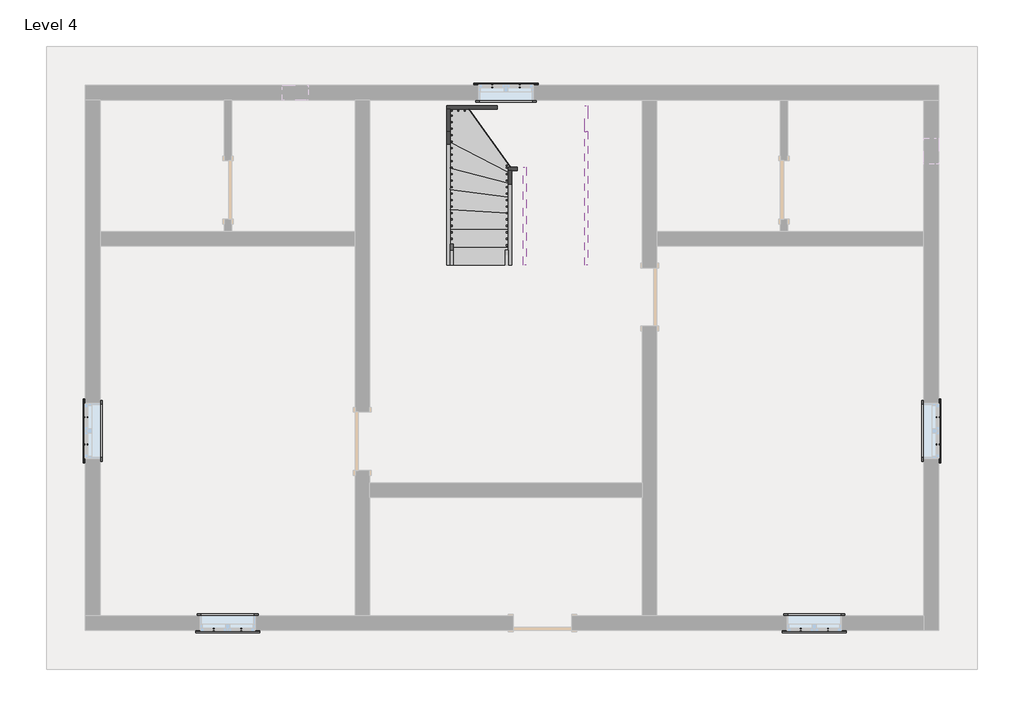
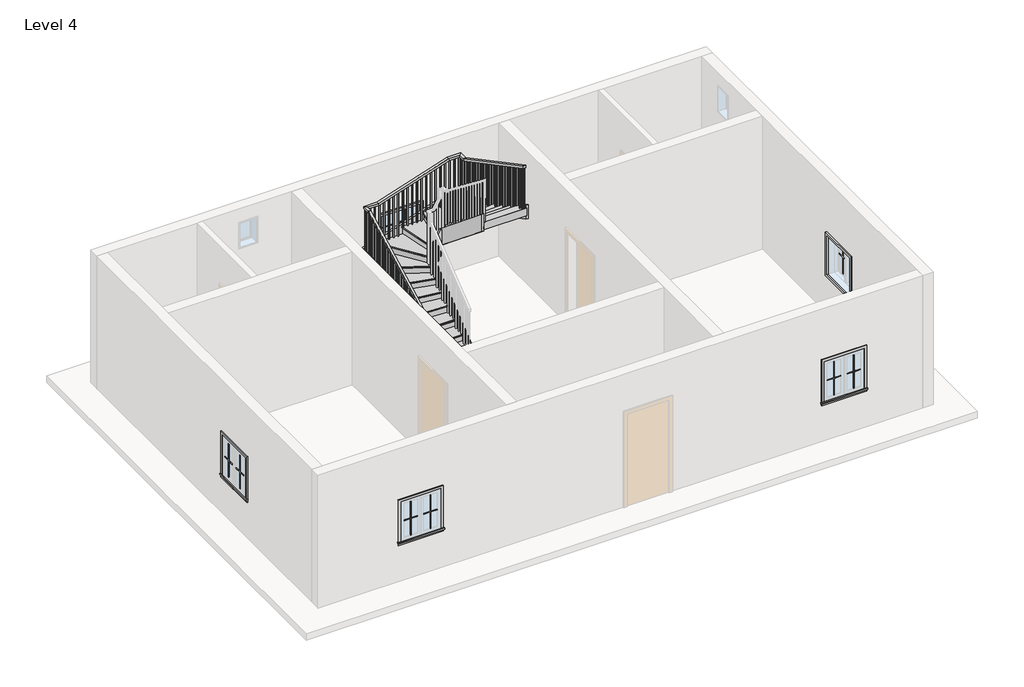
# One storey, part 2 of 2: 20 proxies, 8 members, 1 railing, 1 stair flight.
"""IFC4 building model written with IfcOpenShell, lengths in millimetres."""

from ifc_helpers import new_model, si_unit, frame, origin, place, context, project, spatial, polyline, outline, extrude, faceted_brep, transform, mapped, element, save
from components import muntin_pattern_2x2_muntin_pattern_2x2_b3fe6957, muntin_pattern_2x2_muntin_pattern_2x2_3e0ecaf2, trim_window_exterior_flat_with_sill_41619996, trim_window_interior_flat_picture_frame_51c85655, stair_flight_9737d4c8

model = new_model("IFC4")

# Units and contexts
model_context = context("Model", 3, world=origin())
ifc_project = project(units=[si_unit("LENGTHUNIT", "METRE", prefix="MILLI")], contexts=[model_context])

# Site, building, storey
site = spatial("IfcSite", under=ifc_project)
building = spatial("IfcBuilding", under=site)
storey = spatial("IfcBuildingStorey", under=building, Name="Level 4", Elevation=6400.8)

# Proxies
placement = place(None, origin())
muntin_pattern_2x2_muntin_pattern_2x2_shape = muntin_pattern_2x2_muntin_pattern_2x2_b3fe6957(model_context)
element("IfcBuildingElementProxy", 1, Name="Muntin Pattern_2x2 : Muntin Pattern_2x2", ObjectType="Muntin Pattern_2x2 : Muntin Pattern_2x2", at=placement, inside=storey, context=model_context, shape_type="MappedRepresentation", body=[
    mapped(muntin_pattern_2x2_muntin_pattern_2x2_shape, transform((-7325.4390964, 833.891032, 7385.05), x_axis=(0.0, 1.0, 0.0), y_axis=(-1.0, 0.0, 0.0), z_axis=(0.0, 0.0, 1.0))),
])
element("IfcBuildingElementProxy", 2, Name="Muntin Pattern_2x2 : Muntin Pattern_2x2", ObjectType="Muntin Pattern_2x2 : Muntin Pattern_2x2", at=placement, inside=storey, context=model_context, shape_type="MappedRepresentation", body=[
    mapped(muntin_pattern_2x2_muntin_pattern_2x2_shape, transform((6006.3859036, 1262.516032, 7385.05), x_axis=(0.0, -1.0, 0.0), y_axis=(1.0, 0.0, 0.0), z_axis=(0.0, 0.0, 1.0))),
])
element("IfcBuildingElementProxy", 3, Name="Muntin Pattern_2x2 : Muntin Pattern_2x2", ObjectType="Muntin Pattern_2x2 : Muntin Pattern_2x2", at=placement, inside=storey, context=model_context, shape_type="MappedRepresentation", body=[
    mapped(muntin_pattern_2x2_muntin_pattern_2x2_shape, transform((-967.5015964, 6448.878532, 7385.05), x_axis=(1.0, 0.0, 0.0), y_axis=(0.0, 1.0, 0.0), z_axis=(0.0, 0.0, 1.0))),
])
element("IfcBuildingElementProxy", 4, Name="Muntin Pattern_2x2 : Muntin Pattern_2x2", ObjectType="Muntin Pattern_2x2 : Muntin Pattern_2x2", at=placement, inside=storey, context=model_context, shape_type="MappedRepresentation", body=[
    mapped(muntin_pattern_2x2_muntin_pattern_2x2_shape, transform((-4896.5640964, -2066.471468, 7385.05), x_axis=(-1.0, 0.0, 0.0), y_axis=(0.0, -1.0, 0.0), z_axis=(0.0, 0.0, 1.0))),
])
element("IfcBuildingElementProxy", 5, Name="Muntin Pattern_2x2 : Muntin Pattern_2x2", ObjectType="Muntin Pattern_2x2 : Muntin Pattern_2x2", at=placement, inside=storey, context=model_context, shape_type="MappedRepresentation", body=[
    mapped(muntin_pattern_2x2_muntin_pattern_2x2_shape, transform((4287.1234036, -2066.471468, 7385.05), x_axis=(-1.0, 0.0, 0.0), y_axis=(0.0, -1.0, 0.0), z_axis=(0.0, 0.0, 1.0))),
])
muntin_pattern_2x2_muntin_pattern_2x2_2_shape = muntin_pattern_2x2_muntin_pattern_2x2_3e0ecaf2(model_context)
element("IfcBuildingElementProxy", 6, Name="Muntin Pattern_2x2 : Muntin Pattern_2x2", ObjectType="Muntin Pattern_2x2 : Muntin Pattern_2x2", at=placement, inside=storey, context=model_context, shape_type="MappedRepresentation", body=[
    mapped(muntin_pattern_2x2_muntin_pattern_2x2_2_shape, transform((-7325.4390964, 1262.516032, 7385.05), x_axis=(0.0, -1.0, 0.0), y_axis=(1.0, 0.0, 0.0), z_axis=(0.0, 0.0, 1.0))),
])
element("IfcBuildingElementProxy", 7, Name="Muntin Pattern_2x2 : Muntin Pattern_2x2", ObjectType="Muntin Pattern_2x2 : Muntin Pattern_2x2", at=placement, inside=storey, context=model_context, shape_type="MappedRepresentation", body=[
    mapped(muntin_pattern_2x2_muntin_pattern_2x2_2_shape, transform((6006.3859036, 833.891032, 7385.05), x_axis=(0.0, 1.0, 0.0), y_axis=(-1.0, 0.0, 0.0), z_axis=(0.0, 0.0, 1.0))),
])
element("IfcBuildingElementProxy", 8, Name="Muntin Pattern_2x2 : Muntin Pattern_2x2", ObjectType="Muntin Pattern_2x2 : Muntin Pattern_2x2", at=placement, inside=storey, context=model_context, shape_type="MappedRepresentation", body=[
    mapped(muntin_pattern_2x2_muntin_pattern_2x2_2_shape, transform((-538.8765964, 6448.878532, 7385.05), x_axis=(-1.0, 0.0, 0.0), y_axis=(0.0, -1.0, 0.0), z_axis=(0.0, 0.0, 1.0))),
])
element("IfcBuildingElementProxy", 9, Name="Muntin Pattern_2x2 : Muntin Pattern_2x2", ObjectType="Muntin Pattern_2x2 : Muntin Pattern_2x2", at=placement, inside=storey, context=model_context, shape_type="MappedRepresentation", body=[
    mapped(muntin_pattern_2x2_muntin_pattern_2x2_2_shape, transform((-5325.1890964, -2066.471468, 7385.05), x_axis=(1.0, 0.0, 0.0), y_axis=(0.0, 1.0, 0.0), z_axis=(0.0, 0.0, 1.0))),
])
element("IfcBuildingElementProxy", 10, Name="Muntin Pattern_2x2 : Muntin Pattern_2x2", ObjectType="Muntin Pattern_2x2 : Muntin Pattern_2x2", at=placement, inside=storey, context=model_context, shape_type="MappedRepresentation", body=[
    mapped(muntin_pattern_2x2_muntin_pattern_2x2_2_shape, transform((3858.4984036, -2066.471468, 7385.05), x_axis=(1.0, 0.0, 0.0), y_axis=(0.0, 1.0, 0.0), z_axis=(0.0, 0.0, 1.0))),
])
trim_window_exterior_flat_with_sill_shape = trim_window_exterior_flat_with_sill_41619996(model_context)
element("IfcBuildingElementProxy", 11, Name="Trim-Window-Exterior-Flat : with Sill", ObjectType="Trim-Window-Exterior-Flat : with Sill", at=placement, inside=storey, context=model_context, shape_type="MappedRepresentation", body=[
    mapped(trim_window_exterior_flat_with_sill_shape, transform((-7334.9640964, 1048.203532, 8229.6), x_axis=(0.0, -1.0, 0.0), y_axis=(0.0, 0.0, 1.0), z_axis=(-1.0, 0.0, 0.0))),
])
element("IfcBuildingElementProxy", 12, Name="Trim-Window-Exterior-Flat : with Sill", ObjectType="Trim-Window-Exterior-Flat : with Sill", at=placement, inside=storey, context=model_context, shape_type="MappedRepresentation", body=[
    mapped(trim_window_exterior_flat_with_sill_shape, transform((6015.9109036, 1048.203532, 8229.6), x_axis=(0.0, 1.0, 0.0), y_axis=(0.0, 0.0, 1.0), z_axis=(1.0, 0.0, 0.0))),
])
element("IfcBuildingElementProxy", 13, Name="Trim-Window-Exterior-Flat : with Sill", ObjectType="Trim-Window-Exterior-Flat : with Sill", at=placement, inside=storey, context=model_context, shape_type="MappedRepresentation", body=[
    mapped(trim_window_exterior_flat_with_sill_shape, transform((-753.1890964, 6458.403532, 8229.6), x_axis=(-1.0, 0.0, 0.0), y_axis=(0.0, 0.0, 1.0), z_axis=(0.0, 1.0, 0.0))),
])
element("IfcBuildingElementProxy", 14, Name="Trim-Window-Exterior-Flat : with Sill", ObjectType="Trim-Window-Exterior-Flat : with Sill", at=placement, inside=storey, context=model_context, shape_type="MappedRepresentation", body=[
    mapped(trim_window_exterior_flat_with_sill_shape, transform((-5110.8765964, -2075.996468, 8229.6), x_axis=(1.0, 0.0, 0.0), y_axis=(0.0, 0.0, 1.0), z_axis=(0.0, -1.0, 0.0))),
])
element("IfcBuildingElementProxy", 15, Name="Trim-Window-Exterior-Flat : with Sill", ObjectType="Trim-Window-Exterior-Flat : with Sill", at=placement, inside=storey, context=model_context, shape_type="MappedRepresentation", body=[
    mapped(trim_window_exterior_flat_with_sill_shape, transform((4072.8109036, -2075.996468, 8229.6), x_axis=(1.0, 0.0, 0.0), y_axis=(0.0, 0.0, 1.0), z_axis=(0.0, -1.0, 0.0))),
])
trim_window_interior_flat_picture_frame_shape = trim_window_interior_flat_picture_frame_51c85655(model_context)
element("IfcBuildingElementProxy", 16, Name="Trim-Window-Interior-Flat : Picture Frame", ObjectType="Trim-Window-Interior-Flat : Picture Frame", at=placement, inside=storey, context=model_context, shape_type="MappedRepresentation", body=[
    mapped(trim_window_interior_flat_picture_frame_shape, transform((-7106.3640964, 1048.203532, 8229.6), x_axis=(0.0, 1.0, 0.0), y_axis=(0.0, 0.0, 1.0), z_axis=(1.0, 0.0, 0.0))),
])
element("IfcBuildingElementProxy", 17, Name="Trim-Window-Interior-Flat : Picture Frame", ObjectType="Trim-Window-Interior-Flat : Picture Frame", at=placement, inside=storey, context=model_context, shape_type="MappedRepresentation", body=[
    mapped(trim_window_interior_flat_picture_frame_shape, transform((5787.3109036, 1048.203532, 8229.6), x_axis=(0.0, -1.0, 0.0), y_axis=(0.0, 0.0, 1.0), z_axis=(-1.0, 0.0, 0.0))),
])
element("IfcBuildingElementProxy", 18, Name="Trim-Window-Interior-Flat : Picture Frame", ObjectType="Trim-Window-Interior-Flat : Picture Frame", at=placement, inside=storey, context=model_context, shape_type="MappedRepresentation", body=[
    mapped(trim_window_interior_flat_picture_frame_shape, transform((-753.1890964, 6229.803532, 8229.6), x_axis=(1.0, 0.0, 0.0), y_axis=(0.0, 0.0, 1.0), z_axis=(0.0, -1.0, 0.0))),
])
element("IfcBuildingElementProxy", 19, Name="Trim-Window-Interior-Flat : Picture Frame", ObjectType="Trim-Window-Interior-Flat : Picture Frame", at=placement, inside=storey, context=model_context, shape_type="MappedRepresentation", body=[
    mapped(trim_window_interior_flat_picture_frame_shape, transform((-5110.8765964, -1847.396468, 8229.6), x_axis=(-1.0, 0.0, 0.0), y_axis=(0.0, 0.0, 1.0), z_axis=(0.0, 1.0, 0.0))),
])
element("IfcBuildingElementProxy", 20, Name="Trim-Window-Interior-Flat : Picture Frame", ObjectType="Trim-Window-Interior-Flat : Picture Frame", at=placement, inside=storey, context=model_context, shape_type="MappedRepresentation", body=[
    mapped(trim_window_interior_flat_picture_frame_shape, transform((4072.8109036, -1847.396468, 8229.6), x_axis=(-1.0, 0.0, 0.0), y_axis=(0.0, 0.0, 1.0), z_axis=(0.0, 1.0, 0.0))),
])

# Members
element("IfcMember", 21, ObjectType="Stringer - 2\" Width", at=placement, inside=storey, context=model_context, shape_type="SweptSolid", body=[
    extrude(outline(polyline([(3647.9718401, 6400.8), (3647.9718401, 6630.439954), (5735.3890318, 7706.1956453), (5735.3890318, 7363.300629), (3867.7341577, 6400.8), (3647.9718401, 6400.8)])), frame((-1680.2890964, 0.0, 0.0), z_axis=(1.0, 0.0, 0.0), x_axis=(0.0, 1.0, 0.0)), (0.0, 0.0, 1.0), 50.8),
])
element("IfcMember", 22, ObjectType="Stringer - 2\" Width", at=placement, inside=storey, context=model_context, shape_type="SweptSolid", body=[
    extrude(outline(polyline([(-1629.4890964, 5735.3890318), (-1680.2890964, 5735.3890318), (-1680.2890964, 6090.103532), (-1629.4890964, 6090.103532), (-1629.4890964, 5735.3890318)])), frame((0.0, 0.0, 7363.300629), z_axis=(0.0, 0.0, 1.0), x_axis=(1.0, 0.0, 0.0)), (0.0, 0.0, 1.0), 342.8950162),
])
element("IfcMember", 23, ObjectType="Stringer - 2\" Width", at=placement, inside=storey, context=model_context, shape_type="SweptSolid", body=[
    extrude(outline(polyline([(7689.8952212, -1680.2890964), (7401.3956453, -1680.2890964), (7401.3956453, -1510.7666134), (8039.7682298, 478.7109036), (8370.7972697, 478.7109036), (8370.7972697, 441.7307863), (7689.8952212, -1680.2890964)])), frame((0.0, 6090.103532, 0.0), z_axis=(0.0, 1.0, 0.0), x_axis=(0.0, 0.0, 1.0)), (0.0, 0.0, 1.0), 50.8),
])
element("IfcMember", 24, ObjectType="Stringer - 2\" Width", at=placement, inside=storey, context=model_context, shape_type="SweptSolid", body=[
    extrude(outline(polyline([(478.7109036, 6140.903532), (529.5109036, 6140.903532), (529.5109036, 5735.3890318), (478.7109036, 5735.3890318), (478.7109036, 6140.903532)])), frame((0.0, 0.0, 8050.6904473), z_axis=(0.0, 0.0, 1.0), x_axis=(1.0, 0.0, 0.0)), (0.0, 0.0, 1.0), 320.1068224),
])
element("IfcMember", 25, ObjectType="Stringer - 2\" Width", at=placement, inside=storey, context=model_context, shape_type="SweptSolid", body=[
    extrude(outline(polyline([(5735.3890318, 8370.7972697), (5735.3890318, 8050.6904473), (3647.9718401, 9126.4461385), (3647.9718401, 9446.5529609), (5735.3890318, 8370.7972697)])), frame((478.7109036, 0.0, 0.0), z_axis=(1.0, 0.0, 0.0), x_axis=(0.0, 1.0, 0.0)), (0.0, 0.0, 1.0), 50.8),
])
element("IfcMember", 26, ObjectType="Stringer - 2\" Width", at=placement, inside=storey, context=model_context, shape_type="SweptSolid", body=[
    extrude(outline(polyline([(3647.9718401, 6400.8), (3647.9718401, 6576.9764461), (5124.903532, 7781.218648), (5124.903532, 7387.9410923), (3914.2334847, 6400.8), (3647.9718401, 6400.8)])), frame((-715.0890964, 0.0, 0.0), z_axis=(1.0, 0.0, 0.0), x_axis=(0.0, 1.0, 0.0)), (0.0, 0.0, 1.0), 50.8),
])
element("IfcMember", 27, ObjectType="Stringer - 2\" Width", at=placement, inside=storey, context=model_context, shape_type="SweptSolid", body=[
    extrude(outline(polyline([(7974.0682978, -715.0890964), (7429.3617647, -715.0890964), (7429.3617647, -680.846879), (7761.265107, -486.4890964), (8326.9409689, -486.4890964), (8326.9409689, -508.4519789), (7974.0682978, -715.0890964)])), frame((0.0, 5124.903532, 0.0), z_axis=(0.0, 1.0, 0.0), x_axis=(0.0, 0.0, 1.0)), (0.0, 0.0, 1.0), 50.8),
])
element("IfcMember", 28, ObjectType="Stringer - 2\" Width", at=placement, inside=storey, context=model_context, shape_type="SweptSolid", body=[
    extrude(outline(polyline([(5175.703532, 8326.9409689), (5175.703532, 7933.6634131), (3647.9718401, 9179.3262875), (3647.9718401, 9572.6038432), (5175.703532, 8326.9409689)])), frame((-486.4890964, 0.0, 0.0), z_axis=(1.0, 0.0, 0.0), x_axis=(0.0, 1.0, 0.0)), (0.0, 0.0, 1.0), 50.8),
])

# Railing
element("IfcRailing", 29, ObjectType="Handrail - Rectangular", at=placement, inside=storey, context=model_context, shape_type="SolidModel", body=[
    faceted_brep([(-1629.4890964, 3647.9718401, 7484.5333333), (-1629.4890964, 3647.9718401, 7427.0742652), (-1578.6890964, 3647.9718401, 7427.0742652), (-1578.6890964, 3647.9718401, 7484.5333333), (-1629.4890964, 5905.6969022, 8677.8239201), (-1629.4890964, 5918.2959667, 8627.0239201), (-1578.6890964, 5918.2959667, 8627.0239201), (-1578.6890964, 5905.6969022, 8677.8239201), (-1629.4890964, 6090.103532, 8677.8239201), (-1629.4890964, 6090.103532, 8627.0239201), (-1578.6890964, 6039.303532, 8627.0239201), (-1578.6890964, 6039.303532, 8677.8239201), (-1342.1772142, 6090.103532, 8677.8239201), (-1334.2266381, 6090.103532, 8627.0239201), (-1334.2266381, 6039.303532, 8627.0239201), (-1342.1772142, 6039.303532, 8677.8239201), (191.3990215, 6090.103532, 9169.9094132), (199.3495976, 6090.103532, 9119.1094132), (199.3495976, 6039.303532, 9119.1094132), (191.3990215, 6039.303532, 9169.9094132), (478.7109036, 6090.103532, 9169.9094132), (478.7109036, 6090.103532, 9119.1094132), (427.9109036, 6039.303532, 9119.1094132), (427.9109036, 6039.303532, 9169.9094132), (478.7109036, 5905.6969022, 9169.9094132), (478.7109036, 5893.0978376, 9119.1094132), (427.9109036, 5893.0978376, 9119.1094132), (427.9109036, 5905.6969022, 9169.9094132), (478.7109036, 3647.9718401, 10363.2), (427.9109036, 3647.9718401, 10363.2), (427.9109036, 3647.9718401, 10305.7409318), (478.7109036, 3647.9718401, 10305.7409318)], [[[0, 1, 2, 3]], [[1, 0, 4, 5]], [[2, 1, 5, 6]], [[3, 2, 6, 7]], [[0, 3, 7, 4]], [[5, 4, 8, 9]], [[6, 5, 9, 10]], [[7, 6, 10, 11]], [[4, 7, 11, 8]], [[9, 8, 12, 13]], [[10, 9, 13, 14]], [[11, 10, 14, 15]], [[8, 11, 15, 12]], [[13, 12, 16, 17]], [[14, 13, 17, 18]], [[15, 14, 18, 19]], [[12, 15, 19, 16]], [[17, 16, 20, 21]], [[18, 17, 21, 22]], [[19, 18, 22, 23]], [[16, 19, 23, 20]], [[21, 20, 24, 25]], [[22, 21, 25, 26]], [[23, 22, 26, 27]], [[20, 23, 27, 24]], [[28, 29, 30, 31]], [[25, 24, 28, 31]], [[26, 25, 31, 30]], [[27, 26, 30, 29]], [[24, 27, 29, 28]]]),
    extrude(outline(polyline([(3737.428532, 10258.4597858), (3737.428532, 9279.4666667), (3718.378532, 9279.4666667), (3718.378532, 10268.5284102), (3737.428532, 10258.4597858)])), frame((443.7859036, 0.0, 0.0), z_axis=(1.0, 0.0, 0.0), x_axis=(0.0, 1.0, 0.0)), (0.0, 0.0, 1.0), 19.05),
    extrude(outline(polyline([(3839.028532, 10204.7604556), (3839.028532, 9279.4666667), (3819.978532, 9279.4666667), (3819.978532, 10214.82908), (3839.028532, 10204.7604556)])), frame((443.7859036, 0.0, 0.0), z_axis=(1.0, 0.0, 0.0), x_axis=(0.0, 1.0, 0.0)), (0.0, 0.0, 1.0), 19.05),
    extrude(outline(polyline([(3940.628532, 10151.0611254), (3940.628532, 9110.1333333), (3921.578532, 9110.1333333), (3921.578532, 10161.1297498), (3940.628532, 10151.0611254)])), frame((443.7859036, 0.0, 0.0), z_axis=(1.0, 0.0, 0.0), x_axis=(0.0, 1.0, 0.0)), (0.0, 0.0, 1.0), 19.05),
    extrude(outline(polyline([(4042.228532, 10097.3617952), (4042.228532, 9110.1333333), (4023.178532, 9110.1333333), (4023.178532, 10107.4304196), (4042.228532, 10097.3617952)])), frame((443.7859036, 0.0, 0.0), z_axis=(1.0, 0.0, 0.0), x_axis=(0.0, 1.0, 0.0)), (0.0, 0.0, 1.0), 19.05),
    extrude(outline(polyline([(4143.828532, 10043.662465), (4143.828532, 9110.1333333), (4124.778532, 9110.1333333), (4124.778532, 10053.7310894), (4143.828532, 10043.662465)])), frame((443.7859036, 0.0, 0.0), z_axis=(1.0, 0.0, 0.0), x_axis=(0.0, 1.0, 0.0)), (0.0, 0.0, 1.0), 19.05),
    extrude(outline(polyline([(4245.428532, 9989.9631348), (4245.428532, 8940.8), (4226.378532, 8940.8), (4226.378532, 10000.0317592), (4245.428532, 9989.9631348)])), frame((443.7859036, 0.0, 0.0), z_axis=(1.0, 0.0, 0.0), x_axis=(0.0, 1.0, 0.0)), (0.0, 0.0, 1.0), 19.05),
    extrude(outline(polyline([(4347.028532, 9936.2638046), (4347.028532, 8940.8), (4327.978532, 8940.8), (4327.978532, 9946.332429), (4347.028532, 9936.2638046)])), frame((443.7859036, 0.0, 0.0), z_axis=(1.0, 0.0, 0.0), x_axis=(0.0, 1.0, 0.0)), (0.0, 0.0, 1.0), 19.05),
    extrude(outline(polyline([(4448.628532, 9882.5644744), (4448.628532, 8940.8), (4429.578532, 8940.8), (4429.578532, 9892.6330988), (4448.628532, 9882.5644744)])), frame((443.7859036, 0.0, 0.0), z_axis=(1.0, 0.0, 0.0), x_axis=(0.0, 1.0, 0.0)), (0.0, 0.0, 1.0), 19.05),
    extrude(outline(polyline([(4550.228532, 9828.8651442), (4550.228532, 8771.4666667), (4531.178532, 8771.4666667), (4531.178532, 9838.9337686), (4550.228532, 9828.8651442)])), frame((443.7859036, 0.0, 0.0), z_axis=(1.0, 0.0, 0.0), x_axis=(0.0, 1.0, 0.0)), (0.0, 0.0, 1.0), 19.05),
    extrude(outline(polyline([(4651.828532, 9775.165814), (4651.828532, 8771.4666667), (4632.778532, 8771.4666667), (4632.778532, 9785.2344384), (4651.828532, 9775.165814)])), frame((443.7859036, 0.0, 0.0), z_axis=(1.0, 0.0, 0.0), x_axis=(0.0, 1.0, 0.0)), (0.0, 0.0, 1.0), 19.05),
    extrude(outline(polyline([(4753.428532, 9721.4664838), (4753.428532, 8771.4666667), (4734.378532, 8771.4666667), (4734.378532, 9731.5351082), (4753.428532, 9721.4664838)])), frame((443.7859036, 0.0, 0.0), z_axis=(1.0, 0.0, 0.0), x_axis=(0.0, 1.0, 0.0)), (0.0, 0.0, 1.0), 19.05),
    extrude(outline(polyline([(4855.028532, 9667.7671536), (4855.028532, 8602.1333333), (4835.978532, 8602.1333333), (4835.978532, 9677.835778), (4855.028532, 9667.7671536)])), frame((443.7859036, 0.0, 0.0), z_axis=(1.0, 0.0, 0.0), x_axis=(0.0, 1.0, 0.0)), (0.0, 0.0, 1.0), 19.05),
    extrude(outline(polyline([(4956.628532, 9614.0678234), (4956.628532, 8602.1333333), (4937.578532, 8602.1333333), (4937.578532, 9624.1364478), (4956.628532, 9614.0678234)])), frame((443.7859036, 0.0, 0.0), z_axis=(1.0, 0.0, 0.0), x_axis=(0.0, 1.0, 0.0)), (0.0, 0.0, 1.0), 19.05),
    extrude(outline(polyline([(5058.228532, 9560.3684932), (5058.228532, 8602.1333333), (5039.178532, 8602.1333333), (5039.178532, 9570.4371176), (5058.228532, 9560.3684932)])), frame((443.7859036, 0.0, 0.0), z_axis=(1.0, 0.0, 0.0), x_axis=(0.0, 1.0, 0.0)), (0.0, 0.0, 1.0), 19.05),
    extrude(outline(polyline([(5159.828532, 9506.669163), (5159.828532, 8602.1333333), (5140.778532, 8602.1333333), (5140.778532, 9516.7377874), (5159.828532, 9506.669163)])), frame((443.7859036, 0.0, 0.0), z_axis=(1.0, 0.0, 0.0), x_axis=(0.0, 1.0, 0.0)), (0.0, 0.0, 1.0), 19.05),
    extrude(outline(polyline([(5261.428532, 9452.9698328), (5261.428532, 8432.8), (5242.378532, 8432.8), (5242.378532, 9463.0384572), (5261.428532, 9452.9698328)])), frame((443.7859036, 0.0, 0.0), z_axis=(1.0, 0.0, 0.0), x_axis=(0.0, 1.0, 0.0)), (0.0, 0.0, 1.0), 19.05),
    extrude(outline(polyline([(5363.028532, 9399.2705026), (5363.028532, 8432.8), (5343.978532, 8432.8), (5343.978532, 9409.339127), (5363.028532, 9399.2705026)])), frame((443.7859036, 0.0, 0.0), z_axis=(1.0, 0.0, 0.0), x_axis=(0.0, 1.0, 0.0)), (0.0, 0.0, 1.0), 19.05),
    extrude(outline(polyline([(5464.628532, 9345.5711724), (5464.628532, 8432.8), (5445.578532, 8432.8), (5445.578532, 9355.6397968), (5464.628532, 9345.5711724)])), frame((443.7859036, 0.0, 0.0), z_axis=(1.0, 0.0, 0.0), x_axis=(0.0, 1.0, 0.0)), (0.0, 0.0, 1.0), 19.05),
    extrude(outline(polyline([(5566.228532, 9291.8718422), (5566.228532, 8432.8), (5547.178532, 8432.8), (5547.178532, 9301.9404666), (5566.228532, 9291.8718422)])), frame((443.7859036, 0.0, 0.0), z_axis=(1.0, 0.0, 0.0), x_axis=(0.0, 1.0, 0.0)), (0.0, 0.0, 1.0), 19.05),
    extrude(outline(polyline([(5667.828532, 9238.172512), (5667.828532, 8263.4666667), (5648.778532, 8263.4666667), (5648.778532, 9248.2411364), (5667.828532, 9238.172512)])), frame((443.7859036, 0.0, 0.0), z_axis=(1.0, 0.0, 0.0), x_axis=(0.0, 1.0, 0.0)), (0.0, 0.0, 1.0), 19.05),
    extrude(outline(polyline([(5769.428532, 9184.4731818), (5769.428532, 8263.4666667), (5750.378532, 8263.4666667), (5750.378532, 9194.5418062), (5769.428532, 9184.4731818)])), frame((443.7859036, 0.0, 0.0), z_axis=(1.0, 0.0, 0.0), x_axis=(0.0, 1.0, 0.0)), (0.0, 0.0, 1.0), 19.05),
    extrude(outline(polyline([(5871.028532, 9130.7738516), (5871.028532, 8263.4666667), (5851.978532, 8263.4666667), (5851.978532, 9140.842476), (5871.028532, 9130.7738516)])), frame((443.7859036, 0.0, 0.0), z_axis=(1.0, 0.0, 0.0), x_axis=(0.0, 1.0, 0.0)), (0.0, 0.0, 1.0), 19.05),
    extrude(outline(polyline([(462.8359036, 5972.628532), (462.8359036, 5953.578532), (443.7859036, 5953.578532), (443.7859036, 5972.628532), (462.8359036, 5972.628532)])), frame((0.0, 0.0, 8263.4666667), z_axis=(0.0, 0.0, 1.0), x_axis=(1.0, 0.0, 0.0)), (0.0, 0.0, 1.0), 855.6427466),
    extrude(outline(polyline([(418.3859036, 6074.228532), (437.4359036, 6074.228532), (437.4359036, 6055.178532), (418.3859036, 6055.178532), (418.3859036, 6074.228532)])), frame((0.0, 0.0, 8263.4666667), z_axis=(0.0, 0.0, 1.0), x_axis=(1.0, 0.0, 0.0)), (0.0, 0.0, 1.0), 855.6427466),
    extrude(outline(polyline([(316.7859036, 6074.228532), (335.8359036, 6074.228532), (335.8359036, 6055.178532), (316.7859036, 6055.178532), (316.7859036, 6074.228532)])), frame((0.0, 0.0, 8263.4666667), z_axis=(0.0, 0.0, 1.0), x_axis=(1.0, 0.0, 0.0)), (0.0, 0.0, 1.0), 855.6427466),
    extrude(outline(polyline([(215.1859036, 6074.228532), (234.2359036, 6074.228532), (234.2359036, 6055.178532), (215.1859036, 6055.178532), (215.1859036, 6074.228532)])), frame((0.0, 0.0, 8263.4666667), z_axis=(0.0, 0.0, 1.0), x_axis=(1.0, 0.0, 0.0)), (0.0, 0.0, 1.0), 855.6427466),
    extrude(outline(polyline([(9091.5900316, 113.5859036), (8094.1333333, 113.5859036), (8094.1333333, 132.6359036), (9097.7026907, 132.6359036), (9091.5900316, 113.5859036)])), frame((0.0, 6055.178532, 0.0), z_axis=(0.0, 1.0, 0.0), x_axis=(0.0, 0.0, 1.0)), (0.0, 0.0, 1.0), 19.05),
    extrude(outline(polyline([(9058.9891834, 11.9859036), (8094.1333333, 11.9859036), (8094.1333333, 31.0359036), (9065.1018425, 31.0359036), (9058.9891834, 11.9859036)])), frame((0.0, 6055.178532, 0.0), z_axis=(0.0, 1.0, 0.0), x_axis=(0.0, 0.0, 1.0)), (0.0, 0.0, 1.0), 19.05),
    extrude(outline(polyline([(9026.3883352, -89.6140964), (8094.1333333, -89.6140964), (8094.1333333, -70.5640964), (9032.5009942, -70.5640964), (9026.3883352, -89.6140964)])), frame((0.0, 6055.178532, 0.0), z_axis=(0.0, 1.0, 0.0), x_axis=(0.0, 0.0, 1.0)), (0.0, 0.0, 1.0), 19.05),
    extrude(outline(polyline([(8993.787487, -191.2140964), (8094.1333333, -191.2140964), (8094.1333333, -172.1640964), (8999.900146, -172.1640964), (8993.787487, -191.2140964)])), frame((0.0, 6055.178532, 0.0), z_axis=(0.0, 1.0, 0.0), x_axis=(0.0, 0.0, 1.0)), (0.0, 0.0, 1.0), 19.05),
    extrude(outline(polyline([(8961.1866387, -292.8140964), (8094.1333333, -292.8140964), (8094.1333333, -273.7640964), (8967.2992978, -273.7640964), (8961.1866387, -292.8140964)])), frame((0.0, 6055.178532, 0.0), z_axis=(0.0, 1.0, 0.0), x_axis=(0.0, 0.0, 1.0)), (0.0, 0.0, 1.0), 19.05),
    extrude(outline(polyline([(8928.5857905, -394.4140964), (7924.8, -394.4140964), (7924.8, -375.3640964), (8934.6984495, -375.3640964), (8928.5857905, -394.4140964)])), frame((0.0, 6055.178532, 0.0), z_axis=(0.0, 1.0, 0.0), x_axis=(0.0, 0.0, 1.0)), (0.0, 0.0, 1.0), 19.05),
    extrude(outline(polyline([(8895.9849423, -496.0140964), (7924.8, -496.0140964), (7924.8, -476.9640964), (8902.0976013, -476.9640964), (8895.9849423, -496.0140964)])), frame((0.0, 6055.178532, 0.0), z_axis=(0.0, 1.0, 0.0), x_axis=(0.0, 0.0, 1.0)), (0.0, 0.0, 1.0), 19.05),
    extrude(outline(polyline([(8863.384094, -597.6140964), (7924.8, -597.6140964), (7924.8, -578.5640964), (8869.4967531, -578.5640964), (8863.384094, -597.6140964)])), frame((0.0, 6055.178532, 0.0), z_axis=(0.0, 1.0, 0.0), x_axis=(0.0, 0.0, 1.0)), (0.0, 0.0, 1.0), 19.05),
    extrude(outline(polyline([(8830.7832458, -699.2140964), (7924.8, -699.2140964), (7924.8, -680.1640964), (8836.8959049, -680.1640964), (8830.7832458, -699.2140964)])), frame((0.0, 6055.178532, 0.0), z_axis=(0.0, 1.0, 0.0), x_axis=(0.0, 0.0, 1.0)), (0.0, 0.0, 1.0), 19.05),
    extrude(outline(polyline([(8798.1823976, -800.8140964), (7924.8, -800.8140964), (7924.8, -781.7640964), (8804.2950566, -781.7640964), (8798.1823976, -800.8140964)])), frame((0.0, 6055.178532, 0.0), z_axis=(0.0, 1.0, 0.0), x_axis=(0.0, 0.0, 1.0)), (0.0, 0.0, 1.0), 19.05),
    extrude(outline(polyline([(8765.5815494, -902.4140964), (7755.4666667, -902.4140964), (7755.4666667, -883.3640964), (8771.6942084, -883.3640964), (8765.5815494, -902.4140964)])), frame((0.0, 6055.178532, 0.0), z_axis=(0.0, 1.0, 0.0), x_axis=(0.0, 0.0, 1.0)), (0.0, 0.0, 1.0), 19.05),
    extrude(outline(polyline([(8732.9807011, -1004.0140964), (7755.4666667, -1004.0140964), (7755.4666667, -984.9640964), (8739.0933602, -984.9640964), (8732.9807011, -1004.0140964)])), frame((0.0, 6055.178532, 0.0), z_axis=(0.0, 1.0, 0.0), x_axis=(0.0, 0.0, 1.0)), (0.0, 0.0, 1.0), 19.05),
    extrude(outline(polyline([(8700.3798529, -1105.6140964), (7755.4666667, -1105.6140964), (7755.4666667, -1086.5640964), (8706.492512, -1086.5640964), (8700.3798529, -1105.6140964)])), frame((0.0, 6055.178532, 0.0), z_axis=(0.0, 1.0, 0.0), x_axis=(0.0, 0.0, 1.0)), (0.0, 0.0, 1.0), 19.05),
    extrude(outline(polyline([(8667.7790047, -1207.2140964), (7755.4666667, -1207.2140964), (7755.4666667, -1188.1640964), (8673.8916637, -1188.1640964), (8667.7790047, -1207.2140964)])), frame((0.0, 6055.178532, 0.0), z_axis=(0.0, 1.0, 0.0), x_axis=(0.0, 0.0, 1.0)), (0.0, 0.0, 1.0), 19.05),
    extrude(outline(polyline([(8635.1781565, -1308.8140964), (7755.4666667, -1308.8140964), (7755.4666667, -1289.7640964), (8641.2908155, -1289.7640964), (8635.1781565, -1308.8140964)])), frame((0.0, 6055.178532, 0.0), z_axis=(0.0, 1.0, 0.0), x_axis=(0.0, 0.0, 1.0)), (0.0, 0.0, 1.0), 19.05),
    extrude(outline(polyline([(-1410.4140964, 6074.228532), (-1391.3640964, 6074.228532), (-1391.3640964, 6055.178532), (-1410.4140964, 6055.178532), (-1410.4140964, 6074.228532)])), frame((0.0, 0.0, 7586.1333333), z_axis=(0.0, 0.0, 1.0), x_axis=(1.0, 0.0, 0.0)), (0.0, 0.0, 1.0), 1040.8905868),
    extrude(outline(polyline([(-1512.0140964, 6074.228532), (-1492.9640964, 6074.228532), (-1492.9640964, 6055.178532), (-1512.0140964, 6055.178532), (-1512.0140964, 6074.228532)])), frame((0.0, 0.0, 7586.1333333), z_axis=(0.0, 0.0, 1.0), x_axis=(1.0, 0.0, 0.0)), (0.0, 0.0, 1.0), 1040.8905868),
    extrude(outline(polyline([(-1613.6140964, 5975.2468401), (-1613.6140964, 5994.2968401), (-1594.5640964, 5994.2968401), (-1594.5640964, 5975.2468401), (-1613.6140964, 5975.2468401)])), frame((0.0, 0.0, 7586.1333333), z_axis=(0.0, 0.0, 1.0), x_axis=(1.0, 0.0, 0.0)), (0.0, 0.0, 1.0), 1040.8905868),
    extrude(outline(polyline([(5892.6968401, 8613.4938418), (5892.6968401, 7586.1333333), (5873.6468401, 7586.1333333), (5873.6468401, 8603.4252174), (5892.6968401, 8613.4938418)])), frame((-1613.6140964, 0.0, 0.0), z_axis=(1.0, 0.0, 0.0), x_axis=(0.0, 1.0, 0.0)), (0.0, 0.0, 1.0), 19.05),
    extrude(outline(polyline([(5791.0968401, 8559.7945116), (5791.0968401, 7586.1333333), (5772.0468401, 7586.1333333), (5772.0468401, 8549.7258872), (5791.0968401, 8559.7945116)])), frame((-1613.6140964, 0.0, 0.0), z_axis=(1.0, 0.0, 0.0), x_axis=(0.0, 1.0, 0.0)), (0.0, 0.0, 1.0), 19.05),
    extrude(outline(polyline([(5689.4968401, 8506.0951814), (5689.4968401, 7586.1333333), (5670.4468401, 7586.1333333), (5670.4468401, 8496.026557), (5689.4968401, 8506.0951814)])), frame((-1613.6140964, 0.0, 0.0), z_axis=(1.0, 0.0, 0.0), x_axis=(0.0, 1.0, 0.0)), (0.0, 0.0, 1.0), 19.05),
    extrude(outline(polyline([(5587.8968401, 8452.3958512), (5587.8968401, 7586.1333333), (5568.8468401, 7586.1333333), (5568.8468401, 8442.3272268), (5587.8968401, 8452.3958512)])), frame((-1613.6140964, 0.0, 0.0), z_axis=(1.0, 0.0, 0.0), x_axis=(0.0, 1.0, 0.0)), (0.0, 0.0, 1.0), 19.05),
    extrude(outline(polyline([(5486.2968401, 8398.696521), (5486.2968401, 7416.8), (5467.2468401, 7416.8), (5467.2468401, 8388.6278966), (5486.2968401, 8398.696521)])), frame((-1613.6140964, 0.0, 0.0), z_axis=(1.0, 0.0, 0.0), x_axis=(0.0, 1.0, 0.0)), (0.0, 0.0, 1.0), 19.05),
    extrude(outline(polyline([(5384.6968401, 8344.9971908), (5384.6968401, 7416.8), (5365.6468401, 7416.8), (5365.6468401, 8334.9285664), (5384.6968401, 8344.9971908)])), frame((-1613.6140964, 0.0, 0.0), z_axis=(1.0, 0.0, 0.0), x_axis=(0.0, 1.0, 0.0)), (0.0, 0.0, 1.0), 19.05),
    extrude(outline(polyline([(5283.0968401, 8291.2978606), (5283.0968401, 7416.8), (5264.0468401, 7416.8), (5264.0468401, 8281.2292362), (5283.0968401, 8291.2978606)])), frame((-1613.6140964, 0.0, 0.0), z_axis=(1.0, 0.0, 0.0), x_axis=(0.0, 1.0, 0.0)), (0.0, 0.0, 1.0), 19.05),
    extrude(outline(polyline([(5181.4968401, 8237.5985304), (5181.4968401, 7416.8), (5162.4468401, 7416.8), (5162.4468401, 8227.529906), (5181.4968401, 8237.5985304)])), frame((-1613.6140964, 0.0, 0.0), z_axis=(1.0, 0.0, 0.0), x_axis=(0.0, 1.0, 0.0)), (0.0, 0.0, 1.0), 19.05),
    extrude(outline(polyline([(5079.8968401, 8183.8992002), (5079.8968401, 7247.4666667), (5060.8468401, 7247.4666667), (5060.8468401, 8173.8305758), (5079.8968401, 8183.8992002)])), frame((-1613.6140964, 0.0, 0.0), z_axis=(1.0, 0.0, 0.0), x_axis=(0.0, 1.0, 0.0)), (0.0, 0.0, 1.0), 19.05),
    extrude(outline(polyline([(4978.2968401, 8130.19987), (4978.2968401, 7247.4666667), (4959.2468401, 7247.4666667), (4959.2468401, 8120.1312456), (4978.2968401, 8130.19987)])), frame((-1613.6140964, 0.0, 0.0), z_axis=(1.0, 0.0, 0.0), x_axis=(0.0, 1.0, 0.0)), (0.0, 0.0, 1.0), 19.05),
    extrude(outline(polyline([(4876.6968401, 8076.5005398), (4876.6968401, 7247.4666667), (4857.6468401, 7247.4666667), (4857.6468401, 8066.4319154), (4876.6968401, 8076.5005398)])), frame((-1613.6140964, 0.0, 0.0), z_axis=(1.0, 0.0, 0.0), x_axis=(0.0, 1.0, 0.0)), (0.0, 0.0, 1.0), 19.05),
    extrude(outline(polyline([(4775.0968401, 8022.8012096), (4775.0968401, 7078.1333333), (4756.0468401, 7078.1333333), (4756.0468401, 8012.7325852), (4775.0968401, 8022.8012096)])), frame((-1613.6140964, 0.0, 0.0), z_axis=(1.0, 0.0, 0.0), x_axis=(0.0, 1.0, 0.0)), (0.0, 0.0, 1.0), 19.05),
    extrude(outline(polyline([(4673.4968401, 7969.1018794), (4673.4968401, 7078.1333333), (4654.4468401, 7078.1333333), (4654.4468401, 7959.033255), (4673.4968401, 7969.1018794)])), frame((-1613.6140964, 0.0, 0.0), z_axis=(1.0, 0.0, 0.0), x_axis=(0.0, 1.0, 0.0)), (0.0, 0.0, 1.0), 19.05),
    extrude(outline(polyline([(4571.8968401, 7915.4025492), (4571.8968401, 7078.1333333), (4552.8468401, 7078.1333333), (4552.8468401, 7905.3339248), (4571.8968401, 7915.4025492)])), frame((-1613.6140964, 0.0, 0.0), z_axis=(1.0, 0.0, 0.0), x_axis=(0.0, 1.0, 0.0)), (0.0, 0.0, 1.0), 19.05),
    extrude(outline(polyline([(4470.2968401, 7861.703219), (4470.2968401, 6908.8), (4451.2468401, 6908.8), (4451.2468401, 7851.6345946), (4470.2968401, 7861.703219)])), frame((-1613.6140964, 0.0, 0.0), z_axis=(1.0, 0.0, 0.0), x_axis=(0.0, 1.0, 0.0)), (0.0, 0.0, 1.0), 19.05),
    extrude(outline(polyline([(4368.6968401, 7808.0038888), (4368.6968401, 6908.8), (4349.6468401, 6908.8), (4349.6468401, 7797.9352644), (4368.6968401, 7808.0038888)])), frame((-1613.6140964, 0.0, 0.0), z_axis=(1.0, 0.0, 0.0), x_axis=(0.0, 1.0, 0.0)), (0.0, 0.0, 1.0), 19.05),
    extrude(outline(polyline([(4267.0968401, 7754.3045586), (4267.0968401, 6908.8), (4248.0468401, 6908.8), (4248.0468401, 7744.2359342), (4267.0968401, 7754.3045586)])), frame((-1613.6140964, 0.0, 0.0), z_axis=(1.0, 0.0, 0.0), x_axis=(0.0, 1.0, 0.0)), (0.0, 0.0, 1.0), 19.05),
    extrude(outline(polyline([(4165.4968401, 7700.6052284), (4165.4968401, 6739.4666667), (4146.4468401, 6739.4666667), (4146.4468401, 7690.536604), (4165.4968401, 7700.6052284)])), frame((-1613.6140964, 0.0, 0.0), z_axis=(1.0, 0.0, 0.0), x_axis=(0.0, 1.0, 0.0)), (0.0, 0.0, 1.0), 19.05),
    extrude(outline(polyline([(4063.8968401, 7646.9058982), (4063.8968401, 6739.4666667), (4044.8468401, 6739.4666667), (4044.8468401, 7636.8372738), (4063.8968401, 7646.9058982)])), frame((-1613.6140964, 0.0, 0.0), z_axis=(1.0, 0.0, 0.0), x_axis=(0.0, 1.0, 0.0)), (0.0, 0.0, 1.0), 19.05),
    extrude(outline(polyline([(3962.2968401, 7593.206568), (3962.2968401, 6739.4666667), (3943.2468401, 6739.4666667), (3943.2468401, 7583.1379436), (3962.2968401, 7593.206568)])), frame((-1613.6140964, 0.0, 0.0), z_axis=(1.0, 0.0, 0.0), x_axis=(0.0, 1.0, 0.0)), (0.0, 0.0, 1.0), 19.05),
    extrude(outline(polyline([(3860.6968401, 7539.5072378), (3860.6968401, 6570.1333333), (3841.6468401, 6570.1333333), (3841.6468401, 7529.4386134), (3860.6968401, 7539.5072378)])), frame((-1613.6140964, 0.0, 0.0), z_axis=(1.0, 0.0, 0.0), x_axis=(0.0, 1.0, 0.0)), (0.0, 0.0, 1.0), 19.05),
    extrude(outline(polyline([(3759.0968401, 7485.8079076), (3759.0968401, 6570.1333333), (3740.0468401, 6570.1333333), (3740.0468401, 7475.7392831), (3759.0968401, 7485.8079076)])), frame((-1613.6140964, 0.0, 0.0), z_axis=(1.0, 0.0, 0.0), x_axis=(0.0, 1.0, 0.0)), (0.0, 0.0, 1.0), 19.05),
    extrude(outline(polyline([(443.7859036, 6074.228532), (462.8359036, 6074.228532), (462.8359036, 6055.178532), (443.7859036, 6055.178532), (443.7859036, 6074.228532)])), frame((0.0, 0.0, 8263.4666667), z_axis=(0.0, 0.0, 1.0), x_axis=(1.0, 0.0, 0.0)), (0.0, 0.0, 1.0), 855.6427466),
    extrude(outline(polyline([(-1613.6140964, 6055.178532), (-1613.6140964, 6074.228532), (-1594.5640964, 6074.228532), (-1594.5640964, 6055.178532), (-1613.6140964, 6055.178532)])), frame((0.0, 0.0, 7586.1333333), z_axis=(0.0, 0.0, 1.0), x_axis=(1.0, 0.0, 0.0)), (0.0, 0.0, 1.0), 1040.8905868),
    extrude(outline(polyline([(3667.0218401, 10295.6723074), (3667.0218401, 9279.4666667), (3647.9718401, 9279.4666667), (3647.9718401, 10305.7409318), (3667.0218401, 10295.6723074)])), frame((443.7859036, 0.0, 0.0), z_axis=(1.0, 0.0, 0.0), x_axis=(0.0, 1.0, 0.0)), (0.0, 0.0, 1.0), 19.05),
    extrude(outline(polyline([(3667.0218401, 7437.1428896), (3667.0218401, 6570.1333333), (3647.9718401, 6570.1333333), (3647.9718401, 7427.0742652), (3667.0218401, 7437.1428896)])), frame((-1613.6140964, 0.0, 0.0), z_axis=(1.0, 0.0, 0.0), x_axis=(0.0, 1.0, 0.0)), (0.0, 0.0, 1.0), 19.05),
])

# Stair flight
stair_flight_shape = stair_flight_9737d4c8(model_context)
element("IfcStairFlight", 30, ObjectType="2\" Tread 1\" Nosing 1/4\" Riser", at=placement, inside=storey, context=model_context, shape_type="MappedRepresentation", body=[
    mapped(stair_flight_shape, transform((0.0, 0.0, 0.0), x_axis=(1.0, 0.0, 0.0), y_axis=(0.0, 1.0, 0.0), z_axis=(0.0, 0.0, 1.0))),
])

save(model, "model.ifc")

# Revit data of these elements
# Type "Muntin Pattern_2x2 : Muntin Pattern_2x2"
#   Width [instance default] = 4' - 0"
#   Thickness = 0' - 0 1/2"
#   Height [instance default] = 4' - 0"
#   Distance = 0' - 0 3/4"
#   Interior Material [instance default] = none
#   Exterior Material [instance default] = none
#   Default Elevation = 0
# Type "Trim-Window-Exterior-Flat : with Sill"
#   Trim Width = 0' - 2 1/4"
#   Trim Thickness_Picture Frame = 0' - 1 1/4"
#   Trim Thickness_with Sill = 0' - 0 3/4"
#   Sill Thickness = 0' - 1 1/4"
#   Opening Width [instance default] = 2' - 0"
#   Opening Height [instance default] = 3' - 0"
#   Default Elevation = 4' - 0"
#   Sill = yes
#   Picture Frame = no
#   Trim Material [instance default] = none
# Type "Trim-Window-Interior-Flat : Picture Frame"
#   Trim Thickness_Picture Frame = 0' - 1 1/4"
#   Trim Width = 0' - 2 1/4"
#   Trim Thickness_with Sill = 0' - 0 3/4"
#   Sill Thickness = 0' - 1 1/4"
#   Opening Width [instance default] = 2' - 0"
#   Opening Height [instance default] = 3' - 0"
#   Default Elevation = 4' - 0"
#   Sill = no
#   Picture Frame = yes
#   Trim Material [instance default] = none
# Type "Handrail - Rectangular"
#   Assembly Code = "C2010400"
#   built-in parameter 1008612 = 0.0416667 (stored number, unit not read)
#   built-in parameter 1008611 = 0.0416667 (stored number, unit not read)
#   built-in parameter 1008609 = 0.333333 (stored number, unit not read)
#   built-in parameter 1008604 = 0.166667 (stored number, unit not read)
#   built-in parameter 1008603 = 0.166667 (stored number, unit not read)
#   Railing Height = 3' - 0"
#   built-in parameter 1008630 = 2
#   built-in parameter 1008610 = 2
#   built-in parameter 1008618 = Baluster - Square : 3/4"
# Elements 1, 2, 3, 4, 5, 6, 7, 8, 9, 10 (IfcBuildingElementProxy, "Muntin Pattern_2x2 : Muntin Pattern_2x2")
#   Width = 0' - 11 5/8"
#   Height = 2' - 6 1/2"
#   Interior Material = Wood - Stained
#   Exterior Material = Clad - White
#   Phase Created = New Construction
#   Materials on its faces: "Clad - White", "Wood - Stained"
# Elements 11, 12, 13, 14, 15 (IfcBuildingElementProxy, "Trim-Window-Exterior-Flat : with Sill")
#   Opening Width = 2' - 10"
#   Opening Height = 3' - 0"
#   Trim Material = Clad - White
#   Phase Created = New Construction
#   Materials on its faces: "Clad - White"
# Elements 16, 17, 18, 19, 20 (IfcBuildingElementProxy, "Trim-Window-Interior-Flat : Picture Frame")
#   Opening Width = 2' - 10"
#   Opening Height = 3' - 0"
#   Trim Material = Wood - Stained
#   Phase Created = New Construction
#   Materials on its faces: "Wood - Stained"
# Elements 21, 22, 23, 24, 25, 26, 27, 28 (IfcMember, "Stringer - 2\" Width")
#   Phase Created = New Construction
# Element 29 (IfcRailing, "Handrail - Rectangular")
#   Phase Created = New Construction
# Element 30 (IfcStairFlight, "2\" Tread 1\" Nosing 1/4\" Riser")
#   Phase Created = New Construction
# Materials
#   "Clad - White": class "Wood", colour RGB 242 242 238, transparency 0, Cost = 0
#   "Wood - Stained": class "Wood", colour RGB 224 178 126, transparency 0, Cost = 0
